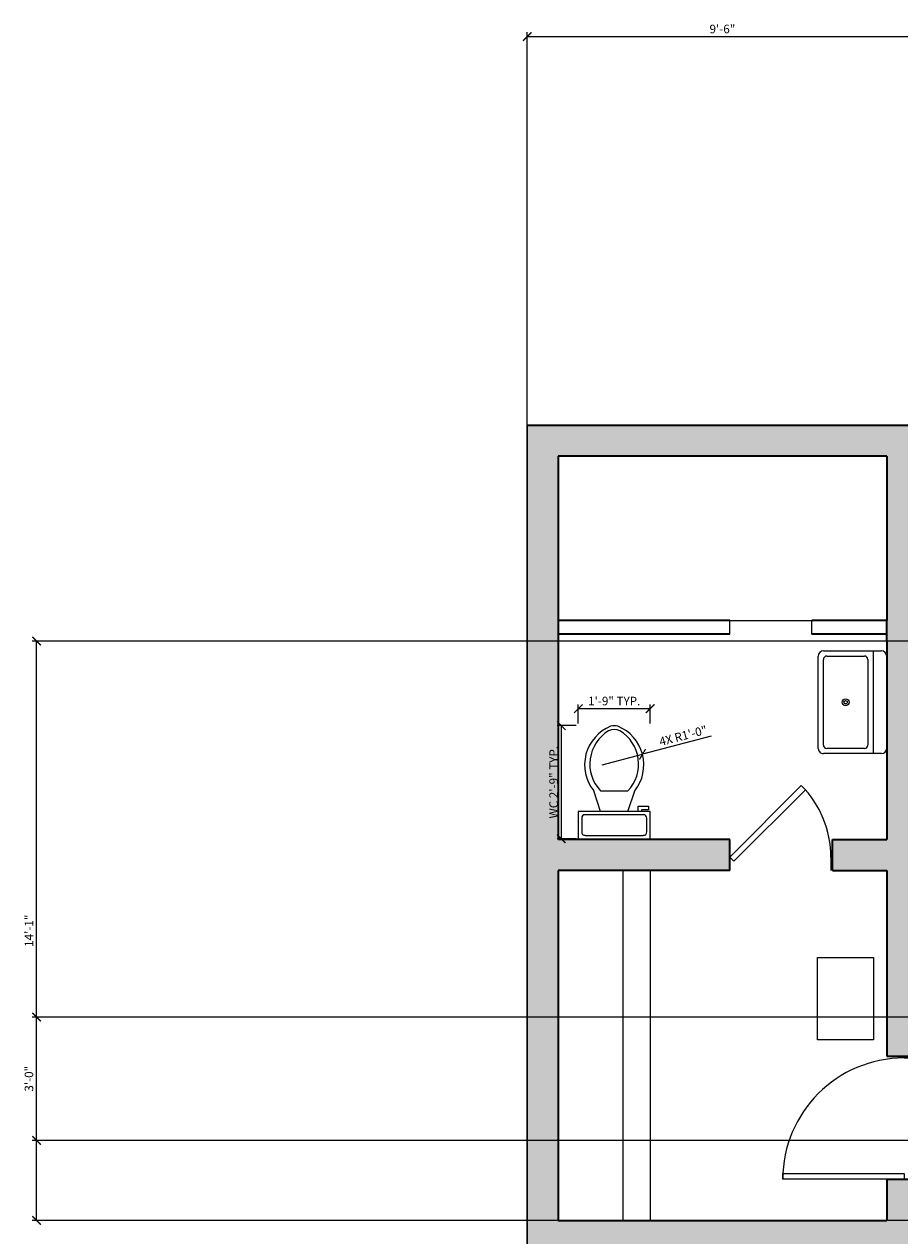
# Model space of a CAD drawing. Units: inches. Extents: x 3122 to 5933, y 1474 to 2995.
# Tile 8 of 12: x 4918 to 5174, y 2639 to 2993. Entities that reach past the tile are written whole.
import ezdxf

# ---------------------------------------------------------------- set-up
doc = ezdxf.new("R2010")
doc.units = ezdxf.units.IN
for name, color, linetype, lineweight in [('A-ANNO-DIMS', 2, 'Continuous', 18), ('A-DOOR', 4, 'Continuous', 25), ('A-FLOR-CASE', 8, 'Continuous', 18), ('A-FLOR-FIXT', 9, 'Continuous', 18), ('A-FURN', 8, 'Continuous', 18), ('A-GLAZ', 4, 'Continuous', 18), ('A-WALL', 7, 'Continuous', 35), ('A-WALL-PATT', 7, 'Continuous', 13), ('C-PROP', 7, 'Continuous', 25)]:
    doc.layers.add(name, color=color, linetype=linetype, lineweight=lineweight)
doc.styles.get("Standard").update_dxf_attribs({"font": 'arial.ttf'})
doc.dimstyles.new('ISO-25', dxfattribs={"dimtxt": 2.5, "dimasz": 2.5, "dimexe": 1.25, "dimexo": 0.625, "dimtad": 1, "dimdec": 0, "dimlunit": 3, "dimtxsty": 'Standard', "dimblk": 'ARCHTICK', "dimcen": 2.5, "dimadec": 0, "dimazin": 0, "dimtfac": 1, "dimtdec": 0, "dimtmove": 0, "dimatfit": 3, "dimfxl": 1, "dimarcsym": 0})

# ---------------------------------------------------------------- blocks, each defined once
blk = doc.blocks.new('*U26')
for p, q in [((0, 0), (0, -100)), ((750, 0), (750, -100))]:
    blk.add_line(p, q)
blk.add_lwpolyline([(0, 0), (530.3, 530.3), (561.3, 499.4), (30.9, -30.9)], close=True)
blk.add_arc((0, 0), 750, 0, 45)
blk = doc.blocks.new('*U25')
for p, q in [((0, 0), (0, -100)), ((900, 0), (900, -100))]:
    blk.add_line(p, q)
blk.add_lwpolyline([(0, 0), (0, 900), (43.75, 900), (43.75, 0)], close=True)
blk.add_arc((0, 0), 900, 0, 90)
blk = doc.blocks.new('Toilet - top')
for p, q in [((9.5, -6), (9.5, -2)), ((-10, -8.5), (-8, -8.5)), ((-10, -9.5), (-10, -8.5)), ((-7, -9.5), (-10, -9.5)), ((-8, -8.5), (-8, -8)), ((-7, -8), (-7, -9.5)), ((-4, -8), (-6, -14)), ((4, -8), (6, -14)), ((4, -14), (-4, -14))]:
    blk.add_line(p, q)
blk.add_lwpolyline([(10.5, -8), (10.5, 0), (-10.5, 0), (-10.5, -8)], close=True)
for points in [[(-9.5, -2), (-9.5, -6)], [(8.5, -1), (-8.5, -1)], [(-8.5, -7), (8.5, -7)]]:
    blk.add_lwpolyline(points)
for centre, radius, start, end in [((-8.62, -1.88), 0.884, 81.8699, 188.1301), ((8.62, -1.88), 0.884, 351.8699, 98.1301), ((-8.62, -6.12), 0.884, 171.8699, 278.1301), ((8.62, -6.12), 0.884, 261.8699, 8.1301), ((3.52, -21.58), 12.17, 141.4691, 247.9714), ((4.2, -21.82), 11.33, 136.3677, 238.9468), ((-3.52, -21.58), 12.17, 292.0284, 38.5307), ((-4.2, -21.82), 11.33, 301.053, 43.6321), ((0, -27.88), 4, 245.7318, 294.2682), ((0, -29), 4, 254.8605, 285.1395)]:
    blk.add_arc(centre, radius, start, end)
blk = doc.blocks.new('Sink-single - 30 in top')
blk.add_line((-15, -3.999996), (15, -3.999996))
for points in [[(-13.5, 0), (13.5, 0)], [(-15, -18.499996), (-15, -1.5)], [(15, -1.5), (15, -18.499996)], [(-13.5, -17.499996), (-13.5, -6.499996)], [(-12.5, -5.499996), (12.5, -5.499996)], [(13.5, -6.499996), (13.5, -17.499996)], [(13.5, -19.999996), (-13.5, -19.999996)], [(12.5, -18.499996), (-12.5, -18.499996)]]:
    blk.add_lwpolyline(points)
for radius in [1, 0.5]:
    blk.add_circle((0, -11.999996), radius)
for centre, radius, start, end in [((-13.5, -1.5), 1.5, 90, 180), ((13.5, -1.5), 1.5, 0, 90), ((-12.5, -6.499996), 1, 90, 180), ((12.5, -6.499996), 1, 0, 90), ((-12.5, -17.499996), 1, 180, 270), ((12.5, -17.499996), 1, 270, 0), ((-13.5, -18.499996), 1.5, 180, 270), ((13.5, -18.499996), 1.5, 270, 0)]:
    blk.add_arc(centre, radius, start, end)
blk = doc.blocks.new('_ArchTick')
at = {"color": 0, "linetype": 'ByBlock', "const_width": 0.15}
blk.add_lwpolyline([(-0.5, -0.5), (0.5, 0.5)], dxfattribs=at)
blk = doc.blocks.new('*D60')
at = {"layer": 'A-ANNO-DIMS', "color": 0, "lineweight": -2, "transparency": 16777216}
for p, q in [((5079.23, 2788.21), (5073.65, 2788.21)), ((5074.9, 2788.21), (5074.9, 2755.16)), ((5079.23, 2755.16), (5073.65, 2755.16))]:
    blk.add_line(p, q, dxfattribs=at)
at = {"layer": 'Defpoints', "color": 0, "transparency": 16777216}
for p in [(5079.86, 2788.21), (5074.9, 2755.16), (5079.86, 2755.16)]:
    blk.add_point(p, dxfattribs=at)
at = {"layer": 'A-ANNO-DIMS', "color": 0, "lineweight": -2, "transparency": 16777216, "xscale": 2.5, "yscale": 2.5, "zscale": 2.5}
for p, rotation in [((5074.9, 2788.21), 90), ((5074.9, 2755.16), 270)]:
    blk.add_blockref('_ArchTick', p, dxfattribs=dict(at, rotation=rotation))
at = {"layer": 'A-ANNO-DIMS', "color": 0, "transparency": 16777216, "insert": (5072.98, 2771.68), "char_height": 2.5, "attachment_point": 5, "rotation": 90}
blk.add_mtext('WC 2\'-9" TYP.', dxfattribs=at)
blk = doc.blocks.new('*D61')
at = {"layer": 'A-ANNO-DIMS', "color": 0, "lineweight": -2, "transparency": 16777216}
for p, q in [((5079.86, 2788.83), (5079.86, 2794.41)), ((5100.86, 2793.16), (5079.86, 2793.16)), ((5100.86, 2788.83), (5100.86, 2794.41))]:
    blk.add_line(p, q, dxfattribs=at)
at = {"layer": 'Defpoints', "color": 0, "transparency": 16777216}
for p in [(5079.86, 2793.16), (5079.86, 2788.21), (5100.86, 2788.21)]:
    blk.add_point(p, dxfattribs=at)
at = {"layer": 'A-ANNO-DIMS', "color": 0, "lineweight": -2, "transparency": 16777216, "xscale": 2.5, "yscale": 2.5, "zscale": 2.5, "rotation": 180}
blk.add_blockref('_ArchTick', (5079.86, 2793.16), dxfattribs=at)
at = {"layer": 'A-ANNO-DIMS', "color": 0, "lineweight": -2, "transparency": 16777216, "xscale": 2.5, "yscale": 2.5, "zscale": 2.5}
blk.add_blockref('_ArchTick', (5100.86, 2793.16), dxfattribs=at)
at = {"layer": 'A-ANNO-DIMS', "color": 0, "transparency": 16777216, "insert": (5090.36, 2795.07), "char_height": 2.5, "attachment_point": 5}
blk.add_mtext('1\'-9" TYP.', dxfattribs=at)
blk = doc.blocks.new('*D94')
at = {"layer": 'A-ANNO-DIMS', "color": 0, "lineweight": -2, "transparency": 16777216}
for p, q in [((5064.96, 1916.52), (5064.96, 2990.75)), ((5487.87, 1916.52), (5487.87, 2990.75)), ((5064.96, 2989.5), (5487.87, 2989.5))]:
    blk.add_line(p, q, dxfattribs=at)
at = {"layer": 'Defpoints', "color": 0, "transparency": 16777216}
for p in [(5487.87, 2989.5), (5064.96, 1915.9), (5487.87, 1915.9)]:
    blk.add_point(p, dxfattribs=at)
at = {"layer": 'A-ANNO-DIMS', "color": 0, "lineweight": -2, "transparency": 16777216, "xscale": 2.5, "yscale": 2.5, "zscale": 2.5, "rotation": 180}
blk.add_blockref('_ArchTick', (5064.96, 2989.5), dxfattribs=at)
at = {"layer": 'A-ANNO-DIMS', "color": 0, "lineweight": -2, "transparency": 16777216, "xscale": 2.5, "yscale": 2.5, "zscale": 2.5}
blk.add_blockref('_ArchTick', (5487.87, 2989.5), dxfattribs=at)
at = {"layer": 'A-ANNO-DIMS', "color": 0, "transparency": 16777216, "insert": (5276.42, 2991.41), "char_height": 2.5, "attachment_point": 5}
blk.add_mtext('35\'-3"', dxfattribs=at)
blk = doc.blocks.new('*D95')
at = {"layer": 'A-ANNO-DIMS', "color": 0, "lineweight": -2, "transparency": 16777216}
for p, q in [((5064.96, 2876.52), (5064.96, 2990.75)), ((5178.96, 2876.52), (5178.96, 2990.75)), ((5064.96, 2989.5), (5178.96, 2989.5))]:
    blk.add_line(p, q, dxfattribs=at)
at = {"layer": 'Defpoints', "color": 0, "transparency": 16777216}
for p in [(5178.96, 2989.5), (5064.96, 2875.9), (5178.96, 2875.9)]:
    blk.add_point(p, dxfattribs=at)
at = {"layer": 'A-ANNO-DIMS', "color": 0, "lineweight": -2, "transparency": 16777216, "xscale": 2.5, "yscale": 2.5, "zscale": 2.5, "rotation": 180}
blk.add_blockref('_ArchTick', (5064.96, 2989.5), dxfattribs=at)
at = {"layer": 'A-ANNO-DIMS', "color": 0, "lineweight": -2, "transparency": 16777216, "xscale": 2.5, "yscale": 2.5, "zscale": 2.5}
blk.add_blockref('_ArchTick', (5178.96, 2989.5), dxfattribs=at)
at = {"layer": 'A-ANNO-DIMS', "color": 0, "transparency": 16777216, "insert": (5121.96, 2991.4), "char_height": 2.5, "attachment_point": 5}
blk.add_mtext('9\'-6"', dxfattribs=at)
blk = doc.blocks.new('*D109')
at = {"layer": 'A-ANNO-DIMS', "color": 0, "lineweight": -2, "transparency": 16777216}
for p, q in [((5178.34, 2812.9), (4920.36, 2812.9)), ((4921.61, 2643.69), (4921.61, 2812.9)), ((5178.34, 2643.69), (4920.36, 2643.69))]:
    blk.add_line(p, q, dxfattribs=at)
at = {"layer": 'Defpoints', "color": 0, "transparency": 16777216}
for p in [(4921.61, 2812.9), (5178.96, 2812.9), (5178.96, 2643.69)]:
    blk.add_point(p, dxfattribs=at)
at = {"layer": 'A-ANNO-DIMS', "color": 0, "lineweight": -2, "transparency": 16777216, "xscale": 2.5, "yscale": 2.5, "zscale": 2.5}
for p, rotation in [((4921.61, 2812.9), 90), ((4921.61, 2643.69), 270)]:
    blk.add_blockref('_ArchTick', p, dxfattribs=dict(at, rotation=rotation))
at = {"layer": 'A-ANNO-DIMS', "color": 0, "transparency": 16777216, "insert": (4919.73, 2728.29), "char_height": 2.5, "attachment_point": 5, "rotation": 90}
blk.add_mtext('14\'-1"', dxfattribs=at)
blk = doc.blocks.new('*D120')
at = {"layer": 'A-ANNO-DIMS', "color": 0, "lineweight": -2, "transparency": 16777216}
for p, q in [((5481.24, 2703.06), (4920.36, 2703.06)), ((4921.61, 2667.06), (4921.61, 2703.06)), ((5481.24, 2667.06), (4920.36, 2667.06))]:
    blk.add_line(p, q, dxfattribs=at)
at = {"layer": 'Defpoints', "color": 0, "transparency": 16777216}
for p in [(4921.61, 2703.06), (5481.87, 2703.06), (5481.87, 2667.06)]:
    blk.add_point(p, dxfattribs=at)
at = {"layer": 'A-ANNO-DIMS', "color": 0, "lineweight": -2, "transparency": 16777216, "xscale": 2.5, "yscale": 2.5, "zscale": 2.5}
for p, rotation in [((4921.61, 2703.06), 90), ((4921.61, 2667.06), 270)]:
    blk.add_blockref('_ArchTick', p, dxfattribs=dict(at, rotation=rotation))
at = {"layer": 'A-ANNO-DIMS', "color": 0, "transparency": 16777216, "insert": (4919.71, 2685.06), "char_height": 2.5, "attachment_point": 5, "rotation": 90}
blk.add_mtext('3\'-0"', dxfattribs=at)
blk = doc.blocks.new('*D131')
at = {"layer": 'A-ANNO-DIMS', "color": 0, "lineweight": -2, "transparency": 16777216}
for p in [(5118.69, 2785.11), (5086.84, 2776.74)]:
    blk.add_line(p, (5098.61, 2779.83), dxfattribs=at)
at = {"layer": 'Defpoints', "color": 0, "transparency": 16777216}
for p in [(5098.61, 2779.83), (5086.84, 2776.74)]:
    blk.add_point(p, dxfattribs=at)
at = {"layer": 'A-ANNO-DIMS', "color": 0, "lineweight": -2, "transparency": 16777216, "xscale": 2.5, "yscale": 2.5, "zscale": 2.5, "rotation": 194.720257809871}
blk.add_blockref('_ArchTick', (5098.61, 2779.83), dxfattribs=at)
at = {"layer": 'A-ANNO-DIMS', "color": 0, "transparency": 16777216, "insert": (5110.58, 2784.95), "char_height": 2.5, "attachment_point": 5, "rotation": 14.7203}
blk.add_mtext('4X R1\'-0"', dxfattribs=at)

msp = doc.modelspace()

# ---------------------------------------------------------------- hatches: boundary and pattern name
at = {"layer": 'A-WALL-PATT'}
h = msp.add_hatch(color=256, dxfattribs=at)
h.dxf.hatch_style = 1
h.paths.add_polyline_path([(5073.96, 2454.69), (5101.59, 2454.69), (5101.59, 2459.69), (5101.59, 2463.69), (5073.96, 2463.69), (5073.96, 2634.69), (5169.96, 2634.69), (5364.96, 2634.69), (5364.96, 2643.69), (5364.96, 2667.06), (5358.96, 2667.06), (5358.96, 2643.69), (5178.96, 2643.69), (5178.96, 2655.69), (5169.96, 2655.69), (5169.96, 2643.69), (5073.96, 2643.69), (5073.96, 2745.9), (5124.13, 2745.9), (5124.13, 2754.9), (5073.96, 2754.9), (5073.96, 2866.9), (5169.96, 2866.9), (5169.96, 2818.9), (5169.96, 2812.9), (5169.96, 2754.9), (5154.13, 2754.9), (5154.13, 2745.9), (5169.96, 2745.9), (5169.96, 2691.69), (5178.96, 2691.69), (5178.96, 2812.9), (5178.96, 2818.9), (5178.96, 2875.9), (5064.96, 2875.9), (5064.96, 2055.71), (5217.96, 2055.71), (5217.96, 2464.19), (5212.96, 2464.19), (5212.96, 2463.69), (5148.19, 2463.69), (5148.19, 2459.69), (5148.19, 2454.69), (5158.96, 2454.69), (5158.96, 2450.72), (5156.04, 2450.72), (5156.04, 2447.72), (5158.96, 2447.72), (5158.96, 2425.1), (5164.96, 2425.1), (5164.96, 2447.72), (5167.71, 2447.72), (5167.71, 2450.72), (5164.96, 2450.72), (5164.96, 2454.69), (5212.96, 2454.69), (5212.96, 2064.71), (5073.96, 2064.71), (5073.96, 2322.69), (5158.96, 2322.69), (5164.96, 2322.69), (5164.96, 2328.69), (5158.96, 2328.69), (5073.96, 2328.69)])

# ---------------------------------------------------------------- linework, layer by layer
at = {"layer": 'A-FLOR-CASE'}
for p, q in [((5092.89, 2745.9), (5092.89, 2643.69)), ((5100.89, 2745.9), (5100.89, 2643.69))]:
    msp.add_line(p, q, dxfattribs=at)
at = {"layer": 'A-FURN'}
msp.add_lwpolyline([(5149.77, 2720.45), (5166.14, 2720.45), (5166.14, 2696.43), (5149.77, 2696.43)], close=True, dxfattribs=at)
at = {"layer": 'A-GLAZ'}
for p, q in [((5124.13, 2814.9), (5124.13, 2818.9)), ((5124.13, 2818.9), (5148.13, 2818.9)), ((5148.13, 2814.9), (5148.13, 2818.9))]:
    msp.add_line(p, q, dxfattribs=at)
at = {"layer": 'A-WALL'}
for p, q in [((5178.96, 2875.9), (5064.96, 2875.9)), ((5073.96, 2866.9), (5073.96, 2754.9)), ((5169.96, 2866.9), (5073.96, 2866.9)), ((5169.96, 2866.9), (5169.96, 2818.9)), ((5124.13, 2818.9), (5073.96, 2818.9)), ((5169.96, 2818.9), (5148.13, 2818.9)), ((5169.96, 2812.9), (5169.96, 2818.9)), ((5124.13, 2814.9), (5073.96, 2814.9)), ((5169.96, 2814.9), (5148.13, 2814.9)), ((5169.96, 2812.9), (5169.96, 2754.9)), ((5124.13, 2754.9), (5073.96, 2754.9)), ((5124.13, 2745.9), (5124.13, 2754.9)), ((5154.13, 2745.9), (5154.13, 2754.9)), ((5154.13, 2754.9), (5169.96, 2754.9)), ((5124.13, 2745.9), (5073.96, 2745.9)), ((5073.96, 2745.9), (5073.96, 2643.69)), ((5154.13, 2745.9), (5169.96, 2745.9)), ((5169.96, 2745.9), (5169.96, 2691.69)), ((5169.96, 2691.69), (5178.96, 2691.69)), ((5169.96, 2655.69), (5178.96, 2655.69)), ((5169.96, 2655.69), (5169.96, 2643.69)), ((5073.96, 2643.69), (5169.96, 2643.69))]:
    msp.add_line(p, q, dxfattribs=at)
at = {"layer": 'C-PROP'}
msp.add_line((5064.96, 2875.9), (5064.96, 1915.9), dxfattribs=at)

# ---------------------------------------------------------------- block references
at = {"layer": 'A-DOOR', "xscale": 0.0393700787401575, "yscale": 0.0393700787401575, "zscale": 0.0393700787401575}
msp.add_blockref('*U26', (5124.13, 2749.83), dxfattribs=at)
at = {"layer": 'A-DOOR', "xscale": 0.0393700787401575, "yscale": 0.0393700787401575, "zscale": 0.0393700787401575, "rotation": 90}
msp.add_blockref('*U25', (5175.03, 2655.69), dxfattribs=at)
at = {"layer": 'A-FLOR-FIXT'}
for name, p, rotation in [('Sink-single - 30 in top', (5169.96, 2795.05), 270), ('Toilet - top', (5090.36, 2755.16), 180)]:
    msp.add_blockref(name, p, dxfattribs=dict(at, rotation=rotation))

# ---------------------------------------------------------------- dimensions: what is measured, and where the dimension line sits
at = {"layer": 'A-ANNO-DIMS'}
for base, p1, p2, picture, middle in [((5487.87, 2989.5), (5064.96, 1915.9), (5487.87, 1915.9), '*D94', (5276.42, 2991.41)), ((5178.96, 2989.5), (5064.96, 2875.9), (5178.96, 2875.9), '*D95', (5121.96, 2991.4))]:
    dim = msp.add_linear_dim(base=base, p1=p1, p2=p2, dimstyle='ISO-25', override={"dimdec": 1, "dimlfac": 1, "dimrnd": 0, "dimzin": 1, "dimdsep": 46, "dimlunit": 4, "dimfrac": 2}, dxfattribs=at)
    dim.commit()
    dim.dimension.update_dxf_attribs({"geometry": picture, "text_midpoint": middle})
for base, p1, p2, picture, middle in [((4921.61, 2812.9), (5178.96, 2643.69), (5178.96, 2812.9), '*D109', (4919.73, 2728.29)), ((4921.61, 2703.06), (5481.87, 2667.06), (5481.87, 2703.06), '*D120', (4919.71, 2685.06))]:
    dim = msp.add_linear_dim(base=base, p1=p1, p2=p2, angle=90, dimstyle='ISO-25', override={"dimdec": 1, "dimlfac": 1, "dimrnd": 0, "dimzin": 1, "dimdsep": 46, "dimlunit": 4, "dimfrac": 2}, dxfattribs=at)
    dim.commit()
    dim.dimension.update_dxf_attribs({"geometry": picture, "text_midpoint": middle})
for base, p1, p2, angle, text, picture, middle in [((5079.86, 2793.16), (5100.86, 2788.21), (5079.86, 2788.21), 180, '<> TYP.', '*D61', (5090.36, 2795.07)), ((5074.9007, 2755.1613), (5079.8576, 2788.2075), (5079.8576, 2755.1613), 270, 'WC <> TYP.', '*D60', (5072.9831, 2771.6844))]:
    dim = msp.add_linear_dim(base=base, p1=p1, p2=p2, angle=angle, text=text, dimstyle='ISO-25', override={"dimdec": 1, "dimlfac": 1, "dimrnd": 0, "dimzin": 1, "dimdsep": 46, "dimlunit": 4, "dimfrac": 2}, dxfattribs=at)
    dim.commit()
    dim.dimension.update_dxf_attribs({"geometry": picture, "text_midpoint": middle})
dim = msp.add_radius_dim(center=(5086.84, 2776.74), mpoint=(5098.61, 2779.83), text='4X <>', dimstyle='ISO-25', override={"dimdec": 1, "dimlfac": 1, "dimrnd": 0, "dimzin": 1, "dimdsep": 46, "dimlunit": 4, "dimfrac": 2}, dxfattribs=at)
dim.commit()
dim.dimension.update_dxf_attribs({"geometry": '*D131', "text_midpoint": (5110.58, 2784.95)})

doc.saveas('drawing.dxf')
